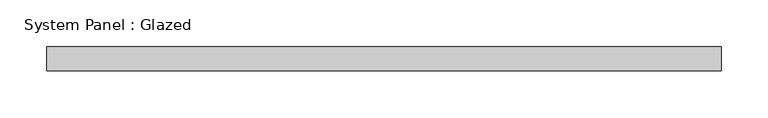
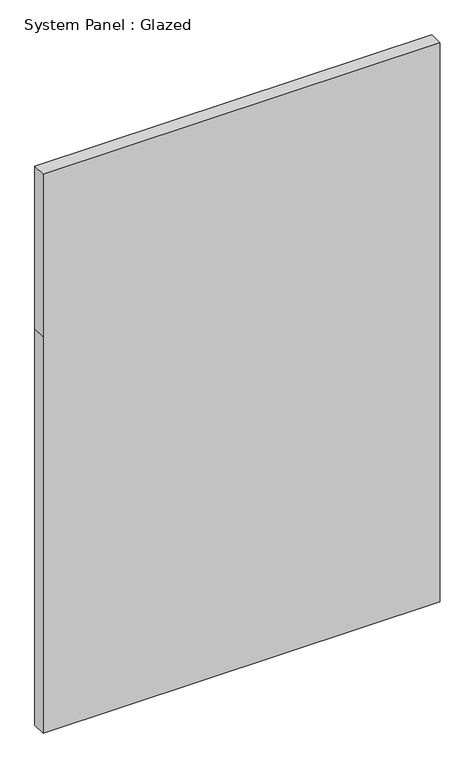
"""IFC4 building model written with IfcOpenShell, lengths in millimetres: plate geometry, System Panel : Glazed."""

from ifc_helpers import new_model, si_unit, frame, origin, place, context, project, spatial, polyline, outline, extrude, source, transform, mapped, element, save


def system_panel_glazed_f4f40b1b(model_context):
    return source(origin(), model_context, "Body", "SweptSolid", [
        extrude(outline(polyline([(0.0, -358.775), (0.0, 358.775), (756.8881029, 358.775), (1066.9664792, 358.775), (1066.9664792, -358.775), (756.8881029, -358.775), (0.0, -358.775)])), frame((0.0, 19.05, 0.0), z_axis=(0.0, 1.0, 0.0), x_axis=(0.0, 0.0, 1.0)), (0.0, 0.0, 1.0), 25.4),
    ])


if __name__ == "__main__":
    model = new_model("IFC4")
    model_context = context("Model", 3, world=origin())
    ifc_project = project(units=[si_unit("LENGTHUNIT", "METRE", prefix="MILLI")], contexts=[model_context])
    site = spatial("IfcSite", under=ifc_project)
    building = spatial("IfcBuilding", under=site)
    placement = place(None, origin())
    system_panel_glazed_shape = system_panel_glazed_f4f40b1b(model_context)
    element("IfcPlate", 1, ObjectType="System Panel : Glazed", at=placement, inside=building, context=model_context, shape_type="MappedRepresentation", body=[
        mapped(system_panel_glazed_shape, transform((0.0, 0.0, 0.0), x_axis=(1.0, 0.0, 0.0), y_axis=(0.0, 1.0, 0.0), z_axis=(0.0, 0.0, 1.0))),
    ])
    save(model, "model.ifc")

# Revit data of these elements
# Type "System Panel : Glazed"
#   Construction Type Id = "GSP4R"
#   Analytic Construction = "1/8 in Pilkington single glazing"
#   Visual Light Transmittance = 0.9
#   Solar Heat Gain Coefficient = 0.86
#   Heat Transfer Coefficient (U) = 1.18115 BTU/(h·ft²·°F)
#   Define Thermal Properties by = 1
# Element 1 (IfcPlate, "System Panel : Glazed")
#   Materials on its faces: "Glass"
# Materials
#   "Glass": class "Glass", colour RGB 0 128 192, transparency 0.75, Description = "Soda Lime Glass", Cost = 0
